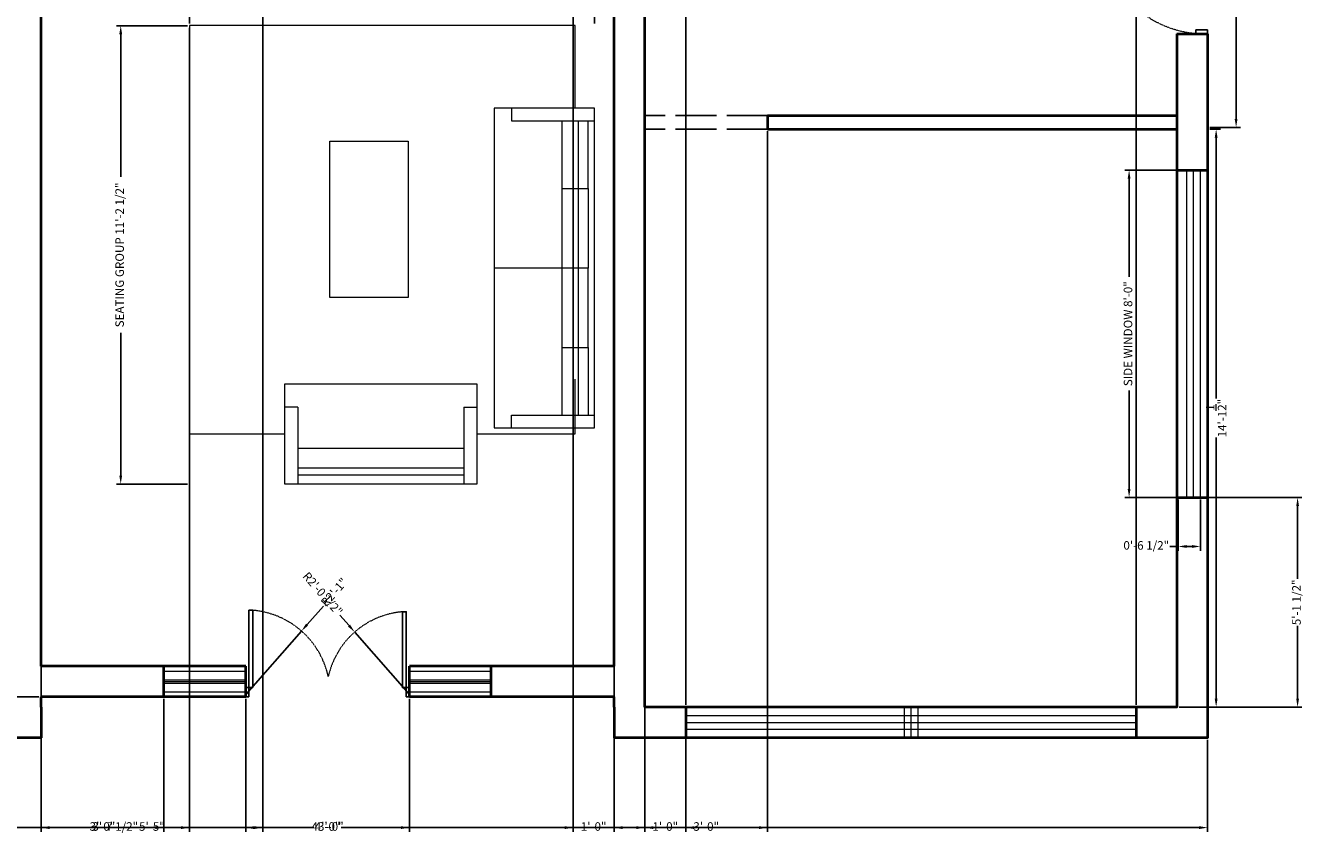
# Model space of a CAD drawing. Units: inches. Extents: x 3502 to 4078, y 3147 to 3541.
# Tile 2 of 3: x 3702 to 4078, y 3147 to 3386. Entities that reach past the tile are written whole.
import ezdxf

# ---------------------------------------------------------------- set-up
doc = ezdxf.new("R2010")
doc.units = ezdxf.units.IN
doc.linetypes.add('ACAD_ISO02W100', pattern=[15, 12, -3])
doc.linetypes.add('HIDDEN4', pattern=[0.09375, 0.0625, -0.03125])
doc.layers.get('0').update_dxf_attribs({"color": 255})
for name, color, linetype, lineweight in [('A-ANNO-DIMS', 2, 'Continuous', 18), ('A-FURN', 8, 'Continuous', 18), ('A-WALL', 7, 'Continuous', 40), ('A-WALL-OVHD', 252, 'ACAD_ISO02W100', 25), ('A-WINDOW', 5, 'Continuous', 15)]:
    doc.layers.add(name, color=color, linetype=linetype, lineweight=lineweight)
doc.layers.add('A-DOOR', color=32, linetype='Continuous', lineweight=25, true_color=0xcd6928)
doc.layers.add('A-DOOR-SWNG', color=32, linetype='HIDDEN4', lineweight=13, true_color=0xcd6928)
doc.styles.get("Standard").update_dxf_attribs({"font": 'arial.ttf'})
doc.dimstyles.new('ISO-25', dxfattribs={"dimtxt": 2.5, "dimasz": 2.5, "dimexe": 1.25, "dimexo": 0.625, "dimtad": 0, "dimlunit": 4, "dimtxsty": 'Standard', "dimcen": 2.5, "dimadec": 0, "dimazin": 0, "dimtfac": 1, "dimtmove": 0, "dimatfit": 3, "dimfxl": 1, "dimarcsym": 0})

# ---------------------------------------------------------------- blocks, each defined once
blk = doc.blocks.new('*D3')
at = {"layer": 'A-ANNO-DIMS', "color": 0, "lineweight": -2, "transparency": 16777216}
for p, q in [((4048.83, 3503.72), (4057.8, 3503.72)), ((4056.55, 3501.22), (4056.55, 3434.53)), ((4056.55, 3358.22), (4056.55, 3424.92)), ((4048.83, 3355.72), (4057.8, 3355.72))]:
    blk.add_line(p, q, dxfattribs=at)
at = {"layer": 'A-ANNO-DIMS', "color": 0, "transparency": 16777216}
for points in [[(4056.13, 3501.22), (4056.96, 3501.22), (4056.55, 3503.72)], [(4056.13, 3358.22), (4056.96, 3358.22), (4056.55, 3355.72)]]:
    blk.add_solid(points, dxfattribs=at)
at = {"layer": 'Defpoints', "color": 0, "transparency": 16777216}
for p in [(4048.21, 3503.72), (4048.21, 3355.72), (4056.55, 3355.72)]:
    blk.add_point(p, dxfattribs=at)
at = {"layer": 'A-ANNO-DIMS', "color": 0, "transparency": 16777216, "insert": (4056.55, 3429.72), "char_height": 2.5, "attachment_point": 5, "rotation": 90}
blk.add_mtext('12\'-4"', dxfattribs=at)
blk = doc.blocks.new('*D4')
at = {"layer": 'A-ANNO-DIMS', "color": 0, "lineweight": -2, "transparency": 16777216}
for p, q in [((4048.83, 3355.22), (4051.95, 3355.22)), ((4050.7, 3352.72), (4050.7, 3276.19)), ((4050.7, 3188.22), (4050.7, 3264.76)), ((4048.83, 3185.72), (4051.95, 3185.72))]:
    blk.add_line(p, q, dxfattribs=at)
at = {"layer": 'A-ANNO-DIMS', "color": 0, "transparency": 16777216}
for points in [[(4050.28, 3352.72), (4051.12, 3352.72), (4050.7, 3355.22)], [(4050.28, 3188.22), (4051.12, 3188.22), (4050.7, 3185.72)]]:
    blk.add_solid(points, dxfattribs=at)
at = {"layer": 'Defpoints', "color": 0, "transparency": 16777216}
for p in [(4048.21, 3355.22), (4050.7, 3355.22), (4048.21, 3185.72)]:
    blk.add_point(p, dxfattribs=at)
at = {"layer": 'A-ANNO-DIMS', "color": 0, "transparency": 16777216, "insert": (4050.7, 3270.47), "char_height": 2.5, "attachment_point": 5, "rotation": 90}
blk.add_mtext('14\'-1{\\H1x;\\S1/2;}"', dxfattribs=at)
blk = doc.blocks.new('A$C5218e9c9')
blk.add_line((50, 6.5), (50, 6.5))
at = {"layer": 'A-WINDOW'}
for p, q in [((0, 4), (96, 4)), ((0, 2), (96, 2)), ((0, 0), (96, 0))]:
    blk.add_line(p, q, dxfattribs=at)
blk = doc.blocks.new('dfglkjdg')
at = {"layer": 'A-DOOR'}
for p, q in [((3245.28, 1353.69), (3245.28, 1357.7)), ((3245.28, 1357.7), (3246.64, 1357.7))]:
    blk.add_line(p, q, dxfattribs=at)
for points in [[(3210.73, 1357.7), (3212.09, 1357.7), (3212.09, 1353.69), (3210.73, 1353.69)], [(3210.73, 1353.69), (3210.73, 1357.7)], [(3245.28, 1353.69), (3246.64, 1353.69), (3246.64, 1357.7)]]:
    blk.add_lwpolyline(points, dxfattribs=at)
blk.add_lwpolyline([(3245.28, 1353.69), (3245.28, 1320.78), (3243.61, 1320.78), (3243.61, 1353.69)], close=True, dxfattribs=at)
at = {"layer": 'A-DOOR-SWNG'}
blk.add_arc((3246.64, 1356.69), 36.04, 184.7792, 265.1785, dxfattribs=at)
blk = doc.blocks.new('SOFA 21')
for p, q in [((-49.09, -24.34), (-49.09, 0)), ((37.16, -24.34), (37.16, 0)), ((-29.27, -1.86), (-49.09, -1.86)), ((-29.27, -9.53), (-29.27, -1.86)), ((-29.27, -1.86), (-5.97, -1.86)), ((17.33, -1.86), (-5.97, -1.86)), ((-5.97, -1.86), (-5.97, -9.53)), ((17.33, -9.53), (17.33, -1.86)), ((17.33, -1.86), (37.16, -1.86)), ((37.16, -4.72), (-49.09, -4.72)), ((37.16, -9.53), (-49.09, -9.53)), ((-5.97, -9.53), (-5.97, -29.38)), ((-52.84, -24.34), (-49.09, -24.34)), ((40.91, -24.34), (37.16, -24.34)), ((-46.78, -38.24), (-46.78, -34.49)), ((-46.78, -38.24), (-69.34, -38.24)), ((-66.74, -38.24), (-66.74, -86.99)), ((-64.62, -86.99), (-64.62, -38.24)), ((-58.88, -38.24), (-58.88, -86.99)), ((-46.78, -86.99), (-69.34, -86.99)), ((-46.78, -86.99), (-46.78, -90.74))]:
    blk.add_line(p, q)
for points in [[(40.91, -29.38), (-52.84, -29.38), (-52.84, 0), (40.91, 0)], [(-69.34, -34.49), (-69.34, -90.74), (-39.97, -90.74), (-39.97, -34.49)]]:
    blk.add_lwpolyline(points, close=True)
at = {"color": 0, "linetype": 'ByBlock', "lineweight": -2}
for points in [[(-54.65, -34.49), (-54.65, -5.62)], [(-54.65, -5.62), (-38.57, -5.62)], [(40.91, -5.62), (65.11, -5.62), (65.11, -118.7), (34.12, -118.7)], [(34.12, -118.7), (-54.65, -118.7), (-54.65, -90.74)]]:
    blk.add_lwpolyline(points, dxfattribs=at)
blk.add_lwpolyline([(-14.65, -77.55), (31.25, -77.55), (31.25, -54.6), (-14.65, -54.6)], close=True, dxfattribs=at)
blk = doc.blocks.new('A$C4f83964a')
blk.add_lwpolyline([(0, 9), (24, 9), (24, 0), (0, 0)], close=True)
at = {"layer": 'A-WINDOW'}
for p, q in [((0, 7.5), (24, 7.5)), ((0, 5), (24, 5)), ((0, 4.5), (24, 4.5)), ((0, 4), (24, 4)), ((0, 1.5), (24, 1.5))]:
    blk.add_line(p, q, dxfattribs=at)
blk = doc.blocks.new('*D21')
at = {"layer": 'A-ANNO-DIMS', "color": 0, "lineweight": -2, "transparency": 16777216}
for p, q in [((4038.95, 3343.22), (4023.93, 3343.22)), ((4025.18, 3340.72), (4025.18, 3311.87)), ((4025.18, 3249.72), (4025.18, 3278.57)), ((4038.95, 3247.22), (4023.93, 3247.22))]:
    blk.add_line(p, q, dxfattribs=at)
at = {"layer": 'A-ANNO-DIMS', "color": 0, "transparency": 16777216}
for points in [[(4024.76, 3340.72), (4025.59, 3340.72), (4025.18, 3343.22)], [(4024.76, 3249.72), (4025.59, 3249.72), (4025.18, 3247.22)]]:
    blk.add_solid(points, dxfattribs=at)
at = {"layer": 'Defpoints', "color": 0, "transparency": 16777216}
for p in [(4025.18, 3343.22), (4039.58, 3343.22), (4039.58, 3247.22)]:
    blk.add_point(p, dxfattribs=at)
at = {"layer": 'A-ANNO-DIMS', "color": 0, "transparency": 16777216, "insert": (4025.18, 3295.22), "char_height": 2.5, "attachment_point": 5, "rotation": 90}
blk.add_mtext('SIDE WINDOW 8\'-0"', dxfattribs=at)
blk = doc.blocks.new('*D22')
at = {"layer": 'A-ANNO-DIMS', "color": 0, "lineweight": -2, "transparency": 16777216}
for p, q in [((4039.58, 3246.6), (4039.58, 3231.57)), ((4046.08, 3246.6), (4046.08, 3231.57)), ((4039.58, 3232.82), (4037.08, 3232.82)), ((4043.58, 3232.82), (4042.08, 3232.82))]:
    blk.add_line(p, q, dxfattribs=at)
at = {"layer": 'A-ANNO-DIMS', "color": 0, "transparency": 16777216}
for points in [[(4042.08, 3233.24), (4042.08, 3232.41), (4039.58, 3232.82)], [(4043.58, 3233.24), (4043.58, 3232.41), (4046.08, 3232.82)]]:
    blk.add_solid(points, dxfattribs=at)
at = {"layer": 'Defpoints', "color": 0, "transparency": 16777216}
for p in [(4039.58, 3247.22), (4046.08, 3247.22), (4039.58, 3232.82)]:
    blk.add_point(p, dxfattribs=at)
at = {"layer": 'A-ANNO-DIMS', "color": 0, "transparency": 16777216, "insert": (4030.22, 3232.82), "char_height": 2.5, "attachment_point": 5}
blk.add_mtext('0\'-6 1/2"', dxfattribs=at)
blk = doc.blocks.new('*D31')
at = {"layer": 'A-ANNO-DIMS', "color": 0, "lineweight": -2, "transparency": 16777216}
for p, q in [((3749.11, 3385.57), (3728.32, 3385.57)), ((3729.57, 3383.07), (3729.57, 3341.21)), ((3729.57, 3253.62), (3729.57, 3295.48)), ((3749.11, 3251.12), (3728.32, 3251.12))]:
    blk.add_line(p, q, dxfattribs=at)
at = {"layer": 'A-ANNO-DIMS', "color": 0, "transparency": 16777216}
for points in [[(3729.15, 3383.07), (3729.98, 3383.07), (3729.57, 3385.57)], [(3729.15, 3253.62), (3729.98, 3253.62), (3729.57, 3251.12)]]:
    blk.add_solid(points, dxfattribs=at)
at = {"layer": 'Defpoints', "color": 0, "transparency": 16777216}
for p in [(3729.57, 3385.57), (3749.73, 3385.57), (3749.73, 3251.12)]:
    blk.add_point(p, dxfattribs=at)
at = {"layer": 'A-ANNO-DIMS', "color": 0, "transparency": 16777216, "insert": (3729.57, 3318.34), "char_height": 2.5, "attachment_point": 5, "rotation": 90}
blk.add_mtext('SEATING GROUP 11\'-2 1/2"', dxfattribs=at)
blk = doc.blocks.new('*D32')
at = {"layer": 'A-ANNO-DIMS', "color": 0, "lineweight": -2, "transparency": 16777216}
for p, q in [((3749.73, 3386.19), (3749.73, 3406.98)), ((3752.23, 3405.73), (3801.25, 3405.73)), ((3865.94, 3405.73), (3816.92, 3405.73)), ((3868.44, 3386.19), (3868.44, 3406.98))]:
    blk.add_line(p, q, dxfattribs=at)
at = {"layer": 'A-ANNO-DIMS', "color": 0, "transparency": 16777216}
for points in [[(3752.23, 3406.15), (3752.23, 3405.32), (3749.73, 3405.73)], [(3865.94, 3406.15), (3865.94, 3405.32), (3868.44, 3405.73)]]:
    blk.add_solid(points, dxfattribs=at)
at = {"layer": 'Defpoints', "color": 0, "transparency": 16777216}
for p in [(3868.44, 3405.73), (3749.73, 3385.57), (3868.44, 3385.57)]:
    blk.add_point(p, dxfattribs=at)
at = {"layer": 'A-ANNO-DIMS', "color": 0, "transparency": 16777216, "insert": (3809.08, 3405.73), "char_height": 2.5, "attachment_point": 5}
blk.add_mtext('9\'-10 1/2"', dxfattribs=at)
blk = doc.blocks.new('*D39')
at = {"layer": 'A-ANNO-DIMS', "color": 0, "lineweight": -2, "transparency": 16777216}
for p, q in [((3706.21, 3503.1), (3706.21, 3149.12)), ((3771.21, 3503.1), (3771.21, 3149.12)), ((3708.71, 3150.37), (3734.76, 3150.37)), ((3768.71, 3150.37), (3742.66, 3150.37))]:
    blk.add_line(p, q, dxfattribs=at)
at = {"layer": 'A-ANNO-DIMS', "color": 0, "transparency": 16777216}
for points in [[(3708.71, 3150.79), (3708.71, 3149.95), (3706.21, 3150.37)], [(3768.71, 3150.79), (3768.71, 3149.95), (3771.21, 3150.37)]]:
    blk.add_solid(points, dxfattribs=at)
at = {"layer": 'Defpoints', "color": 0, "transparency": 16777216}
for p in [(3706.21, 3503.72), (3771.21, 3503.72), (3706.21, 3150.37)]:
    blk.add_point(p, dxfattribs=at)
at = {"layer": 'A-ANNO-DIMS', "color": 0, "transparency": 16777216, "insert": (3738.71, 3150.37), "char_height": 2.5, "attachment_point": 5}
blk.add_mtext('5\'-5"', dxfattribs=at)
blk = doc.blocks.new('*D40')
at = {"layer": 'A-ANNO-DIMS', "color": 0, "lineweight": -2, "transparency": 16777216}
for p, q in [((3862.21, 3503.1), (3862.21, 3149.12)), ((3874.21, 3503.1), (3874.21, 3149.12)), ((3859.71, 3150.37), (3857.21, 3150.37)), ((3862.21, 3150.37), (3864.38, 3150.37)), ((3874.21, 3150.37), (3872.04, 3150.37)), ((3876.71, 3150.37), (3879.21, 3150.37))]:
    blk.add_line(p, q, dxfattribs=at)
at = {"layer": 'A-ANNO-DIMS', "color": 0, "transparency": 16777216}
for points in [[(3859.71, 3150.79), (3859.71, 3149.95), (3862.21, 3150.37)], [(3876.71, 3150.79), (3876.71, 3149.95), (3874.21, 3150.37)]]:
    blk.add_solid(points, dxfattribs=at)
at = {"layer": 'Defpoints', "color": 0, "transparency": 16777216}
for p in [(3862.21, 3503.72), (3874.21, 3503.72), (3874.21, 3150.37)]:
    blk.add_point(p, dxfattribs=at)
at = {"layer": 'A-ANNO-DIMS', "color": 0, "transparency": 16777216, "insert": (3868.21, 3150.37), "char_height": 2.5, "attachment_point": 5}
blk.add_mtext('1\'-0"', dxfattribs=at)
blk = doc.blocks.new('*D43')
at = {"layer": 'A-ANNO-DIMS', "color": 0, "lineweight": -2, "transparency": 16777216}
for p, q in [((3895.21, 3186.35), (3895.21, 3540.35)), ((4027.21, 3186.35), (4027.21, 3540.35)), ((3897.71, 3539.1), (3956.41, 3539.1)), ((4024.71, 3539.1), (3966.01, 3539.1))]:
    blk.add_line(p, q, dxfattribs=at)
at = {"layer": 'A-ANNO-DIMS', "color": 0, "transparency": 16777216}
for points in [[(3897.71, 3539.51), (3897.71, 3538.68), (3895.21, 3539.1)], [(4024.71, 3539.51), (4024.71, 3538.68), (4027.21, 3539.1)]]:
    blk.add_solid(points, dxfattribs=at)
at = {"layer": 'Defpoints', "color": 0, "transparency": 16777216}
for p in [(4027.21, 3539.1), (3895.21, 3185.72), (4027.21, 3185.72)]:
    blk.add_point(p, dxfattribs=at)
at = {"layer": 'A-ANNO-DIMS', "color": 0, "transparency": 16777216, "insert": (3961.21, 3539.1), "char_height": 2.5, "attachment_point": 5}
blk.add_mtext('11\'-0"', dxfattribs=at)
blk = doc.blocks.new('*D44')
at = {"layer": 'A-ANNO-DIMS', "color": 0, "lineweight": -2, "transparency": 16777216}
for p, q in [((3883.21, 3185.09), (3883.21, 3149.12)), ((3895.21, 3185.1), (3895.21, 3149.12)), ((3880.71, 3150.37), (3878.21, 3150.37)), ((3883.21, 3150.37), (3885.38, 3150.37)), ((3895.21, 3150.37), (3893.04, 3150.37)), ((3897.71, 3150.37), (3900.21, 3150.37))]:
    blk.add_line(p, q, dxfattribs=at)
at = {"layer": 'A-ANNO-DIMS', "color": 0, "transparency": 16777216}
for points in [[(3880.71, 3150.79), (3880.71, 3149.95), (3883.21, 3150.37)], [(3897.71, 3150.79), (3897.71, 3149.95), (3895.21, 3150.37)]]:
    blk.add_solid(points, dxfattribs=at)
at = {"layer": 'Defpoints', "color": 0, "transparency": 16777216}
for p in [(3883.21, 3185.72), (3895.21, 3185.72), (3895.21, 3150.37)]:
    blk.add_point(p, dxfattribs=at)
at = {"layer": 'A-ANNO-DIMS', "color": 0, "transparency": 16777216, "insert": (3889.21, 3150.37), "char_height": 2.5, "attachment_point": 5}
blk.add_mtext('1\'-0"', dxfattribs=at)
blk = doc.blocks.new('*D45')
at = {"layer": 'A-ANNO-DIMS', "color": 0, "lineweight": -2, "transparency": 16777216}
for p, q in [((3766.21, 3188.1), (3766.21, 3149.12)), ((3814.21, 3188.1), (3814.21, 3149.12)), ((3768.71, 3150.37), (3786.21, 3150.37)), ((3811.71, 3150.37), (3794.21, 3150.37))]:
    blk.add_line(p, q, dxfattribs=at)
at = {"layer": 'A-ANNO-DIMS', "color": 0, "transparency": 16777216}
for points in [[(3768.71, 3150.79), (3768.71, 3149.95), (3766.21, 3150.37)], [(3811.71, 3150.79), (3811.71, 3149.95), (3814.21, 3150.37)]]:
    blk.add_solid(points, dxfattribs=at)
at = {"layer": 'Defpoints', "color": 0, "transparency": 16777216}
for p in [(3766.21, 3188.72), (3814.21, 3188.72), (3814.21, 3150.37)]:
    blk.add_point(p, dxfattribs=at)
at = {"layer": 'A-ANNO-DIMS', "color": 0, "transparency": 16777216, "insert": (3790.21, 3150.37), "char_height": 2.5, "attachment_point": 5}
blk.add_mtext('4\'-0"', dxfattribs=at)
blk = doc.blocks.new('*D46')
at = {"layer": 'A-ANNO-DIMS', "color": 0, "lineweight": -2, "transparency": 16777216}
for p, q in [((3706.21, 3188.1), (3706.21, 3149.12)), ((3742.21, 3188.1), (3742.21, 3149.12)), ((3708.71, 3150.37), (3720.26, 3150.37)), ((3739.71, 3150.37), (3728.16, 3150.37))]:
    blk.add_line(p, q, dxfattribs=at)
at = {"layer": 'A-ANNO-DIMS', "color": 0, "transparency": 16777216}
for points in [[(3708.71, 3150.79), (3708.71, 3149.95), (3706.21, 3150.37)], [(3739.71, 3150.79), (3739.71, 3149.95), (3742.21, 3150.37)]]:
    blk.add_solid(points, dxfattribs=at)
at = {"layer": 'Defpoints', "color": 0, "transparency": 16777216}
for p in [(3706.21, 3188.72), (3742.21, 3188.72), (3742.21, 3150.37)]:
    blk.add_point(p, dxfattribs=at)
at = {"layer": 'A-ANNO-DIMS', "color": 0, "transparency": 16777216, "insert": (3724.21, 3150.37), "char_height": 2.5, "attachment_point": 5}
blk.add_mtext('3\'-0"', dxfattribs=at)
blk = doc.blocks.new('*D48')
at = {"layer": 'A-ANNO-DIMS', "color": 0, "lineweight": -2, "transparency": 16777216}
for p, q in [((3505.85, 3191.22), (3505.85, 3193.72)), ((3705.58, 3188.72), (3504.6, 3188.72)), ((3505.85, 3188.72), (3505.85, 3186.55)), ((3505.85, 3176.72), (3505.85, 3178.89)), ((3705.58, 3176.72), (3504.6, 3176.72)), ((3505.85, 3174.22), (3505.85, 3171.72))]:
    blk.add_line(p, q, dxfattribs=at)
at = {"layer": 'A-ANNO-DIMS', "color": 0, "transparency": 16777216}
for points in [[(3505.44, 3191.22), (3506.27, 3191.22), (3505.85, 3188.72)], [(3505.44, 3174.22), (3506.27, 3174.22), (3505.85, 3176.72)]]:
    blk.add_solid(points, dxfattribs=at)
at = {"layer": 'Defpoints', "color": 0, "transparency": 16777216}
for p in [(3505.85, 3188.72), (3706.21, 3188.72), (3706.21, 3176.72)]:
    blk.add_point(p, dxfattribs=at)
at = {"layer": 'A-ANNO-DIMS', "color": 0, "transparency": 16777216, "insert": (3505.85, 3182.72), "char_height": 2.5, "attachment_point": 5, "rotation": 90}
blk.add_mtext('1\'-0"', dxfattribs=at)
blk = doc.blocks.new('*D52')
at = {"layer": 'A-ANNO-DIMS', "color": 0, "lineweight": -2, "transparency": 16777216}
for p, q in [((3883.21, 3354.6), (3883.21, 3149.12)), ((3919.21, 3354.6), (3919.21, 3149.12)), ((3885.71, 3150.37), (3897.26, 3150.37)), ((3916.71, 3150.37), (3905.16, 3150.37))]:
    blk.add_line(p, q, dxfattribs=at)
at = {"layer": 'A-ANNO-DIMS', "color": 0, "transparency": 16777216}
for points in [[(3885.71, 3150.79), (3885.71, 3149.95), (3883.21, 3150.37)], [(3916.71, 3150.79), (3916.71, 3149.95), (3919.21, 3150.37)]]:
    blk.add_solid(points, dxfattribs=at)
at = {"layer": 'Defpoints', "color": 0, "transparency": 16777216}
for p in [(3883.21, 3355.22), (3919.21, 3355.22), (3919.21, 3150.37)]:
    blk.add_point(p, dxfattribs=at)
at = {"layer": 'A-ANNO-DIMS', "color": 0, "transparency": 16777216, "insert": (3901.21, 3150.37), "char_height": 2.5, "attachment_point": 5}
blk.add_mtext('3\'-0"', dxfattribs=at)
blk = doc.blocks.new('*D54')
at = {"layer": 'A-ANNO-DIMS', "color": 0, "lineweight": -2, "transparency": 16777216}
for p, q in [((4039.83, 3247.15), (4075.82, 3247.15)), ((4074.57, 3244.65), (4074.57, 3223.3)), ((4074.57, 3188.22), (4074.57, 3209.58)), ((4039.83, 3185.72), (4075.82, 3185.72))]:
    blk.add_line(p, q, dxfattribs=at)
at = {"layer": 'A-ANNO-DIMS', "color": 0, "transparency": 16777216}
for points in [[(4074.16, 3244.65), (4074.99, 3244.65), (4074.57, 3247.15)], [(4074.16, 3188.22), (4074.99, 3188.22), (4074.57, 3185.72)]]:
    blk.add_solid(points, dxfattribs=at)
at = {"layer": 'Defpoints', "color": 0, "transparency": 16777216}
for p in [(4039.21, 3247.15), (4074.57, 3247.15), (4039.21, 3185.72)]:
    blk.add_point(p, dxfattribs=at)
at = {"layer": 'A-ANNO-DIMS', "color": 0, "transparency": 16777216, "insert": (4074.57, 3216.44), "char_height": 2.5, "attachment_point": 5, "rotation": 90}
blk.add_mtext('5\'-1 1/2"', dxfattribs=at)
blk = doc.blocks.new('*D57')
at = {"layer": 'A-ANNO-DIMS', "color": 0, "lineweight": -2, "transparency": 16777216}
for p, q in [((3532.21, 3176.1), (3532.21, 3149.12)), ((4048.21, 3176.1), (4048.21, 3149.12)), ((3534.71, 3150.37), (3785.24, 3150.37)), ((4045.71, 3150.37), (3795.18, 3150.37))]:
    blk.add_line(p, q, dxfattribs=at)
at = {"layer": 'A-ANNO-DIMS', "color": 0, "transparency": 16777216}
for points in [[(3534.71, 3150.79), (3534.71, 3149.95), (3532.21, 3150.37)], [(4045.71, 3150.79), (4045.71, 3149.95), (4048.21, 3150.37)]]:
    blk.add_solid(points, dxfattribs=at)
at = {"layer": 'Defpoints', "color": 0, "transparency": 16777216}
for p in [(3532.21, 3176.72), (4048.21, 3176.72), (4048.21, 3150.37)]:
    blk.add_point(p, dxfattribs=at)
at = {"layer": 'A-ANNO-DIMS', "color": 0, "transparency": 16777216, "insert": (3790.21, 3150.37), "char_height": 2.5, "attachment_point": 5}
blk.add_mtext('43\'-0"', dxfattribs=at)
blk = doc.blocks.new('*D60')
at = {"layer": 'A-ANNO-DIMS', "color": 0, "lineweight": -2, "transparency": 16777216}
for p, q in [((3706.21, 3425.1), (3706.21, 3149.12)), ((3749.73, 3384.94), (3749.73, 3149.12)), ((3708.71, 3150.37), (3721.11, 3150.37)), ((3747.23, 3150.37), (3734.83, 3150.37))]:
    blk.add_line(p, q, dxfattribs=at)
at = {"layer": 'A-ANNO-DIMS', "color": 0, "transparency": 16777216}
for points in [[(3708.71, 3150.79), (3708.71, 3149.95), (3706.21, 3150.37)], [(3747.23, 3150.79), (3747.23, 3149.95), (3749.73, 3150.37)]]:
    blk.add_solid(points, dxfattribs=at)
at = {"layer": 'Defpoints', "color": 0, "transparency": 16777216}
for p in [(3706.21, 3425.72), (3749.73, 3385.57), (3749.73, 3150.37)]:
    blk.add_point(p, dxfattribs=at)
at = {"layer": 'A-ANNO-DIMS', "color": 0, "transparency": 16777216, "insert": (3727.97, 3150.37), "char_height": 2.5, "attachment_point": 5}
blk.add_mtext('3\'-7 1/2"', dxfattribs=at)
blk = doc.blocks.new('*D62')
at = {"layer": 'A-ANNO-DIMS', "color": 0, "lineweight": -2, "transparency": 16777216}
for p, q in [((3788.97, 3215.32), (3784.21, 3209.9)), ((3766.21, 3189.42), (3782.56, 3208.02))]:
    blk.add_line(p, q, dxfattribs=at)
at = {"layer": 'A-ANNO-DIMS', "color": 0, "transparency": 16777216}
blk.add_solid([(3783.89, 3210.18), (3784.52, 3209.63), (3782.56, 3208.02)], dxfattribs=at)
at = {"layer": 'Defpoints', "color": 0, "transparency": 16777216}
for p in [(3782.56, 3208.02), (3766.21, 3189.42)]:
    blk.add_point(p, dxfattribs=at)
at = {"layer": 'A-ANNO-DIMS', "color": 0, "transparency": 16777216, "insert": (3792.37, 3219.19), "char_height": 2.5, "attachment_point": 5, "rotation": 48.6967}
blk.add_mtext('R2\'-1"', dxfattribs=at)
blk = doc.blocks.new('*D63')
at = {"layer": 'A-ANNO-DIMS', "color": 0, "lineweight": -2, "transparency": 16777216}
for p, q in [((3793.85, 3212.65), (3796.51, 3209.61)), ((3814.18, 3189.41), (3798.16, 3207.72))]:
    blk.add_line(p, q, dxfattribs=at)
at = {"layer": 'A-ANNO-DIMS', "color": 0, "transparency": 16777216}
blk.add_solid([(3796.82, 3209.88), (3796.2, 3209.33), (3798.16, 3207.72)], dxfattribs=at)
at = {"layer": 'Defpoints', "color": 0, "transparency": 16777216}
for p in [(3798.16, 3207.72), (3814.18, 3189.41)]:
    blk.add_point(p, dxfattribs=at)
at = {"layer": 'A-ANNO-DIMS', "color": 0, "transparency": 16777216, "insert": (3788.54, 3218.72), "char_height": 2.5, "attachment_point": 5, "rotation": 311.1809}
blk.add_mtext('R2\'-0 1/2"', dxfattribs=at)

msp = doc.modelspace()

# ---------------------------------------------------------------- linework, layer by layer
at = {"layer": 'A-DOOR'}
for p, q in [((3767.145, 3191.482), (3767.145, 3188.724)), ((3813.263, 3191.434), (3813.263, 3188.724)), ((3767.145, 3188.724), (3766.21, 3188.724)), ((3813.263, 3188.724), (3814.182, 3188.724))]:
    msp.add_line(p, q, dxfattribs=at)
for points in [[(3767.145, 3191.482), (3767.145, 3214.097), (3768.292, 3214.097), (3768.292, 3191.482)], [(3813.263, 3191.434), (3813.263, 3213.659), (3812.135, 3213.659), (3812.135, 3191.434)]]:
    msp.add_lwpolyline(points, close=True, dxfattribs=at)
for points in [[(3767.145, 3191.482), (3766.21, 3191.482), (3766.21, 3188.724)], [(3813.263, 3191.434), (3814.182, 3191.434), (3814.182, 3188.724)]]:
    msp.add_lwpolyline(points, dxfattribs=at)
at = {"layer": 'A-DOOR-SWNG'}
for centre, radius, start, end in [((3766.211, 3189.419), 24.766, 12.21274, 85.17852), ((3814.181, 3189.407), 24.338, 94.82148, 167.54051)]:
    msp.add_arc(centre, radius, start, end, dxfattribs=at)
at = {"layer": 'A-WALL'}
for p, q in [((3706.21, 3197.724), (3706.21, 3503.724)), ((3874.21, 3197.724), (3874.21, 3503.724)), ((3883.21, 3359.224), (3883.21, 3503.724)), ((4039.21, 3383.209), (4048.21, 3383.209)), ((3883.21, 3185.72), (3883.21, 3359.224)), ((3919.21, 3359.224), (4039.21, 3359.224)), ((3919.21, 3359.224), (3919.21, 3355.224)), ((3919.21, 3355.224), (4039.21, 3355.224)), ((4039.21, 3343.224), (4048.21, 3343.224)), ((4039.21, 3247.15), (4048.21, 3247.15)), ((3742.21, 3188.724), (3742.21, 3197.724)), ((3766.21, 3188.724), (3766.21, 3197.724)), ((3814.21, 3188.724), (3814.21, 3197.724)), ((3838.21, 3188.724), (3838.21, 3197.724)), ((3706.21, 3185.72), (3706.21, 3188.724)), ((3874.21, 3185.72), (3874.21, 3188.724)), ((3706.21, 3185.724), (3706.21, 3176.724)), ((3874.21, 3185.724), (3874.21, 3176.724)), ((3895.21, 3185.724), (3895.21, 3176.724)), ((4027.21, 3185.724), (4027.21, 3176.724))]:
    msp.add_line(p, q, dxfattribs=at)
for points in [[(4048.21, 3383.209), (4048.21, 3176.724), (3874.21, 3176.724)], [(4039.21, 3383.209), (4039.21, 3185.724), (3883.21, 3185.724)], [(3706.21, 3176.724), (3532.21, 3176.724), (3532.21, 3197.724)], [(3766.21, 3197.724), (3706.21, 3197.724)], [(3874.21, 3197.724), (3814.21, 3197.724)], [(3766.21, 3188.724), (3706.21, 3188.724)], [(3874.21, 3188.724), (3814.21, 3188.724)]]:
    msp.add_lwpolyline(points, dxfattribs=at)
at = {"layer": 'A-WALL-OVHD'}
for p, q in [((3919.21, 3359.224), (3883.21, 3359.224)), ((3919.21, 3355.224), (3883.21, 3355.224))]:
    msp.add_line(p, q, dxfattribs=at)
at = {"layer": 'A-WINDOW'}
for p, q in [((3895.21, 3185.724), (3895.21, 3176.724)), ((3895.21, 3183.224), (4027.21, 3183.224)), ((3959.21, 3185.724), (3959.21, 3176.724)), ((3961.21, 3185.724), (3961.21, 3176.724)), ((3963.21, 3185.724), (3963.21, 3176.724)), ((4027.21, 3185.724), (4027.21, 3176.724)), ((3895.21, 3181.224), (4027.21, 3181.224)), ((3895.21, 3179.224), (4027.21, 3179.224))]:
    msp.add_line(p, q, dxfattribs=at)

# ---------------------------------------------------------------- block references
at = {"layer": 'A-DOOR', "xscale": -0.8352314093545642, "yscale": 0.8352314093545642, "zscale": 0.8352314093545642, "rotation": 270}
msp.add_blockref('dfglkjdg', (2914.129, 701.51), dxfattribs=at)
at = {"layer": 'A-FURN', "xscale": -1, "rotation": 270}
msp.add_blockref('SOFA 21', (3868.435, 3320.462), dxfattribs=at)
at = {"layer": 'A-WINDOW', "rotation": 90}
msp.add_blockref('A$C5218e9c9', (4046.077, 3247.224), dxfattribs=at)
at = {"layer": 'A-WINDOW'}
for p in [(3742.21, 3188.724), (3814.21, 3188.724)]:
    msp.add_blockref('A$C4f83964a', p, dxfattribs=at)

# ---------------------------------------------------------------- dimensions: what is measured, and where the dimension line sits
at = {"layer": 'A-ANNO-DIMS'}
for base, p1, p2, picture, middle in [((4027.21, 3539.096), (3895.21, 3185.724), (4027.21, 3185.724), '*D43', (3961.21, 3539.096)), ((3706.21, 3150.369), (3771.21, 3503.724), (3706.21, 3503.724), '*D39', (3738.71, 3150.369)), ((3874.21, 3150.369), (3862.21, 3503.724), (3874.21, 3503.724), '*D40', (3868.21, 3150.369)), ((3749.732, 3150.369), (3706.21, 3425.724), (3749.732, 3385.567), '*D60', (3727.971, 3150.369)), ((3868.435, 3405.734), (3749.732, 3385.567), (3868.435, 3385.567), '*D32', (3809.084, 3405.734)), ((3919.21, 3150.369), (3883.21, 3355.224), (3919.21, 3355.224), '*D52', (3901.21, 3150.369)), ((3742.21, 3150.369), (3706.21, 3188.724), (3742.21, 3188.724), '*D46', (3724.21, 3150.369)), ((3814.21, 3150.369), (3766.21, 3188.724), (3814.21, 3188.724), '*D45', (3790.21, 3150.369)), ((3895.21, 3150.369), (3883.21, 3185.72), (3895.21, 3185.724), '*D44', (3889.21, 3150.369)), ((4048.21, 3150.369), (3532.21, 3176.724), (4048.21, 3176.724), '*D57', (3790.21, 3150.369))]:
    dim = msp.add_linear_dim(base=base, p1=p1, p2=p2, dimstyle='ISO-25', override={"dimdec": 1, "dimlfac": 1, "dimrnd": 0, "dimzin": 1, "dimdsep": 46, "dimlunit": 4, "dimfrac": 2}, dxfattribs=at)
    dim.commit()
    dim.dimension.update_dxf_attribs({"geometry": picture, "text_midpoint": middle})
for p1, p2, distance, picture, middle in [((4048.21, 3503.724), (4048.21, 3355.724), 8.338, '*D3', (4056.548, 3429.724)), ((4048.21, 3185.724), (4048.21, 3355.224), -2.489, '*D4', (4050.698, 3270.474))]:
    dim = msp.add_aligned_dim(p1=p1, p2=p2, distance=distance, dimstyle='ISO-25', override={"dimclrd": 0, "dimclre": 0, "dimclrt": 0}, dxfattribs=at)
    dim.commit()
    dim.dimension.update_dxf_attribs({"geometry": picture, "text_midpoint": middle})
for base, p1, p2, text, picture, middle in [((3729.565, 3385.567), (3749.732, 3251.12), (3749.732, 3385.567), 'SEATING GROUP <>', '*D31', (3729.565, 3318.344)), ((4025.177, 3343.224), (4039.577, 3247.224), (4039.577, 3343.224), 'SIDE WINDOW <>', '*D21', (4025.177, 3295.224))]:
    dim = msp.add_linear_dim(base=base, p1=p1, p2=p2, angle=90, text=text, dimstyle='ISO-25', override={"dimdec": 1, "dimlfac": 1, "dimrnd": 0, "dimzin": 1, "dimdsep": 46, "dimlunit": 4, "dimfrac": 2}, dxfattribs=at)
    dim.commit()
    dim.dimension.update_dxf_attribs({"geometry": picture, "text_midpoint": middle})
for base, p1, p2, angle, picture, middle in [((4039.577, 3232.824), (4046.077, 3247.224), (4039.577, 3247.224), 180, '*D22', (4030.216, 3232.824)), ((4074.573, 3247.15), (4039.21, 3185.724), (4039.21, 3247.15), 90, '*D54', (4074.573, 3216.437)), ((3505.855, 3188.724), (3706.21, 3176.724), (3706.21, 3188.724), 90, '*D48', (3505.855, 3182.724))]:
    dim = msp.add_linear_dim(base=base, p1=p1, p2=p2, angle=angle, dimstyle='ISO-25', override={"dimdec": 1, "dimlfac": 1, "dimrnd": 0, "dimzin": 1, "dimdsep": 46, "dimlunit": 4, "dimfrac": 2}, dxfattribs=at)
    dim.commit()
    dim.dimension.update_dxf_attribs({"geometry": picture, "text_midpoint": middle})
for center, mpoint, picture, middle in [((3766.211, 3189.419), (3782.557, 3208.023), '*D62', (3792.365, 3219.186)), ((3814.181, 3189.407), (3798.156, 3207.724), '*D63', (3788.541, 3218.715))]:
    dim = msp.add_radius_dim(center=center, mpoint=mpoint, dimstyle='ISO-25', override={"dimdec": 1, "dimlfac": 1, "dimrnd": 0, "dimzin": 1, "dimdsep": 46, "dimlunit": 4, "dimfrac": 2}, dxfattribs=at)
    dim.commit()
    dim.dimension.update_dxf_attribs({"geometry": picture, "text_midpoint": middle, "dimtype": 164})

doc.saveas('drawing.dxf')
